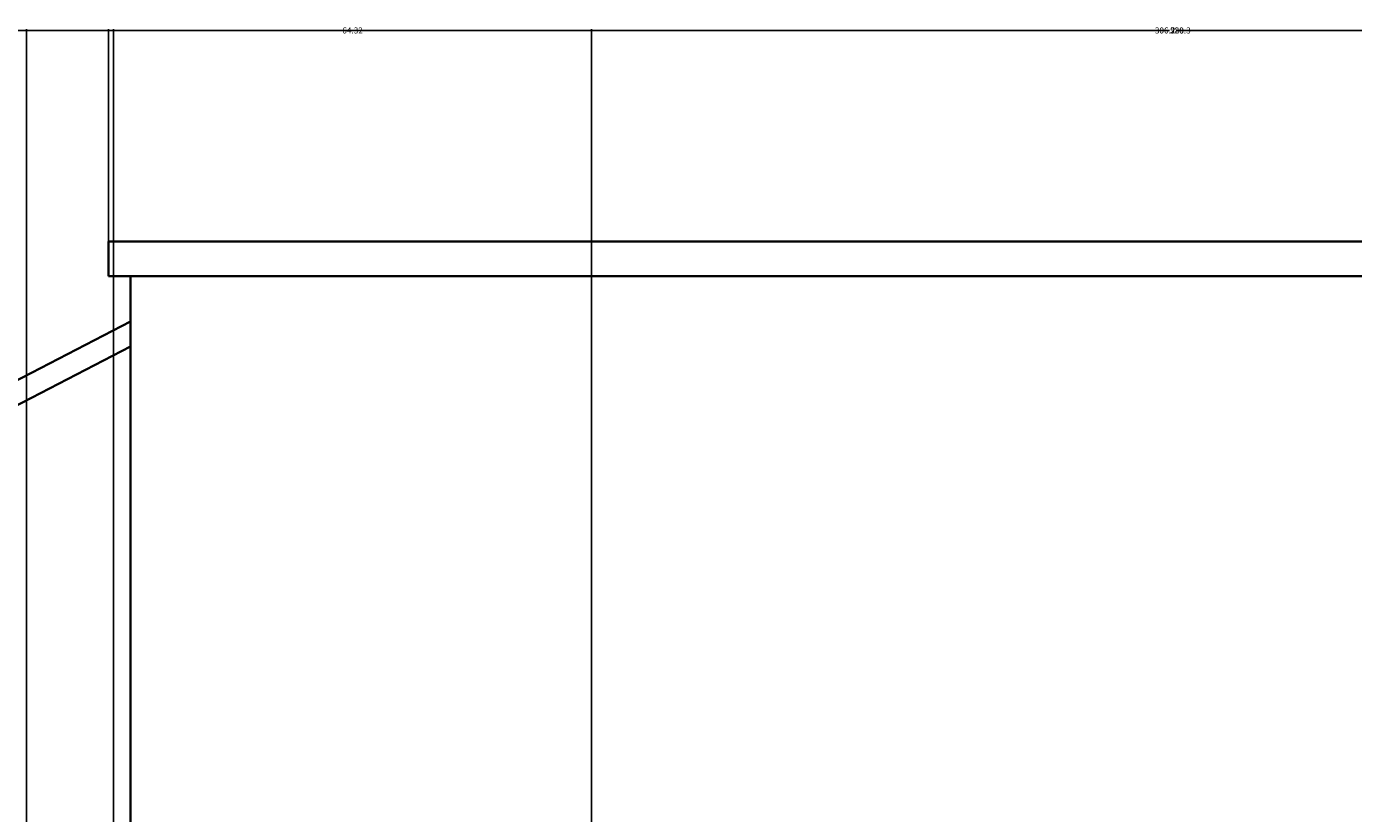
# Model space of a CAD drawing. Units: inches. Extents: x 69 to 650, y -16 to 573.
# Tile 18 of 26: x 205 to 383, y 467 to 573. Entities that reach past the tile are written whole.
import ezdxf

# ---------------------------------------------------------------- set-up
doc = ezdxf.new("R2010")
doc.units = ezdxf.units.IN
doc.header["$MEASUREMENT"] = 0
for name, color, linetype, lineweight in [('A-ANNO-DIMS', 2, 'Continuous', 18), ('A-ROOF', 7, 'Continuous', 35), ('A-WALL', 7, 'Continuous', 35)]:
    doc.layers.add(name, color=color, linetype=linetype, lineweight=lineweight)
doc.styles.get("Standard").update_dxf_attribs({"font": 'arial.ttf'})
doc.dimstyles.get("Standard").update_dxf_attribs({"dimtxt": 0.8125, "dimasz": 0.18, "dimexe": 0.18, "dimexo": 0.0625, "dimgap": 0.09, "dimtad": 0, "dimtih": 1, "dimtoh": 1, "dimdec": 4, "dimzin": 0, "dimdsep": 46, "dimlunit": 4, "dimtxsty": 'Standard', "dimcen": 0.09, "dimadec": 0, "dimazin": 0, "dimtfac": 1, "dimtdec": 4, "dimtofl": 0, "dimtmove": 0, "dimatfit": 3, "dimfxl": 1, "dimtolj": 1, "dimtzin": 0, "dimarcsym": 0})

# ---------------------------------------------------------------- blocks, each defined once
blk = doc.blocks.new('*D19')
at = {"layer": 'A-ANNO-DIMS', "color": 0, "lineweight": -2, "transparency": 16777216}
for p, q in [((99.56, 471.72), (99.56, 572.74)), ((99.74, 572.56), (358.57, 572.56)), ((619.38, 572.56), (360.54, 572.56)), ((619.56, 87.99), (619.56, 572.74))]:
    blk.add_line(p, q, dxfattribs=at)
at = {"layer": 'A-ANNO-DIMS', "color": 0, "transparency": 16777216}
for points in [[(99.74, 572.59), (99.74, 572.53), (99.56, 572.56)], [(619.38, 572.59), (619.38, 572.53), (619.56, 572.56)]]:
    blk.add_solid(points, dxfattribs=at)
at = {"layer": 'Defpoints', "color": 0, "transparency": 16777216}
for p in [(619.56, 572.56), (99.56, 471.66), (619.56, 87.93)]:
    blk.add_point(p, dxfattribs=at)
at = {"layer": 'A-ANNO-DIMS', "color": 0, "transparency": 16777216, "insert": (359.56, 572.56), "char_height": 0.812, "attachment_point": 5}
blk.add_mtext('\\A1;520', dxfattribs=at)
blk = doc.blocks.new('*D45')
at = {"layer": 'A-ANNO-DIMS', "color": 0, "lineweight": -2, "transparency": 16777216}
for p, q in [((216.55, 353.2), (216.55, 572.74)), ((216.73, 572.56), (247.25, 572.56)), ((280.68, 572.56), (250.16, 572.56)), ((280.86, 353.2), (280.86, 572.74))]:
    blk.add_line(p, q, dxfattribs=at)
at = {"layer": 'A-ANNO-DIMS', "color": 0, "transparency": 16777216}
for points in [[(216.73, 572.59), (216.73, 572.53), (216.55, 572.56)], [(280.68, 572.59), (280.68, 572.53), (280.86, 572.56)]]:
    blk.add_solid(points, dxfattribs=at)
at = {"layer": 'Defpoints', "color": 0, "transparency": 16777216}
for p in [(280.86, 572.56), (216.55, 353.14), (280.86, 353.14)]:
    blk.add_point(p, dxfattribs=at)
at = {"layer": 'A-ANNO-DIMS', "color": 0, "transparency": 16777216, "insert": (248.71, 572.56), "char_height": 0.812, "attachment_point": 5}
blk.add_mtext('\\A1;64.32', dxfattribs=at)
blk = doc.blocks.new('*D49')
at = {"layer": 'A-ANNO-DIMS', "color": 0, "lineweight": -2, "transparency": 16777216}
for p, q in [((99.56, 471.72), (99.56, 572.74)), ((99.74, 572.56), (155.98, 572.56)), ((215.7, 572.56), (159.45, 572.56)), ((215.88, 544.22), (215.88, 572.74))]:
    blk.add_line(p, q, dxfattribs=at)
at = {"layer": 'A-ANNO-DIMS', "color": 0, "transparency": 16777216}
for points in [[(99.74, 572.59), (99.74, 572.53), (99.56, 572.56)], [(215.7, 572.59), (215.7, 572.53), (215.88, 572.56)]]:
    blk.add_solid(points, dxfattribs=at)
at = {"layer": 'Defpoints', "color": 0, "transparency": 16777216}
for p in [(215.88, 572.56), (215.88, 544.16), (99.56, 471.66)]:
    blk.add_point(p, dxfattribs=at)
at = {"layer": 'A-ANNO-DIMS', "color": 0, "transparency": 16777216, "insert": (157.72, 572.56), "char_height": 0.812, "attachment_point": 5}
blk.add_mtext('\\A1;116.32', dxfattribs=at)
blk = doc.blocks.new('*D50')
at = {"layer": 'A-ANNO-DIMS', "color": 0, "lineweight": -2, "transparency": 16777216}
for p, q in [((215.88, 544.22), (215.88, 572.74)), ((216.06, 572.56), (358.56, 572.56)), ((504, 572.56), (361.49, 572.56)), ((504.18, 544.22), (504.18, 572.74))]:
    blk.add_line(p, q, dxfattribs=at)
at = {"layer": 'A-ANNO-DIMS', "color": 0, "transparency": 16777216}
for points in [[(216.06, 572.59), (216.06, 572.53), (215.88, 572.56)], [(504, 572.59), (504, 572.53), (504.18, 572.56)]]:
    blk.add_solid(points, dxfattribs=at)
at = {"layer": 'Defpoints', "color": 0, "transparency": 16777216}
for p in [(504.18, 572.56), (215.88, 544.16), (504.18, 544.16)]:
    blk.add_point(p, dxfattribs=at)
at = {"layer": 'A-ANNO-DIMS', "color": 0, "transparency": 16777216, "insert": (360.03, 572.56), "char_height": 0.812, "attachment_point": 5}
blk.add_mtext('\\A1;288.3', dxfattribs=at)
blk = doc.blocks.new('*D62')
at = {"layer": 'A-ANNO-DIMS', "color": 0, "lineweight": -2, "transparency": 16777216}
for p, q in [((204.87, 452.8), (204.87, 572.74)), ((205.05, 572.56), (356.52, 572.56)), ((510.91, 572.56), (359.44, 572.56)), ((511.09, 451.98), (511.09, 572.74))]:
    blk.add_line(p, q, dxfattribs=at)
at = {"layer": 'A-ANNO-DIMS', "color": 0, "transparency": 16777216}
for points in [[(205.05, 572.59), (205.05, 572.53), (204.87, 572.56)], [(510.91, 572.59), (510.91, 572.53), (511.09, 572.56)]]:
    blk.add_solid(points, dxfattribs=at)
at = {"layer": 'Defpoints', "color": 0, "transparency": 16777216}
for p in [(511.09, 572.56), (204.87, 452.74), (511.09, 451.92)]:
    blk.add_point(p, dxfattribs=at)
at = {"layer": 'A-ANNO-DIMS', "color": 0, "transparency": 16777216, "insert": (357.98, 572.56), "char_height": 0.812, "attachment_point": 5}
blk.add_mtext('\\A1;306.2', dxfattribs=at)

msp = doc.modelspace()

# ---------------------------------------------------------------- linework, layer by layer
at = {"layer": 'A-ROOF'}
for p, q in [((215.8767, 539.5075), (215.8767, 544.1573)), ((215.8767, 544.1573), (504.1763, 544.1573)), ((218.848, 539.5075), (215.8767, 539.5075)), ((218.848, 539.5075), (500.263, 539.5075)), ((99.556, 471.6595), (218.848, 533.4142)), ((100.9352, 468.9953), (218.848, 530.036))]:
    msp.add_line(p, q, dxfattribs=at)
at = {"layer": 'A-WALL'}
for p, q in [((218.848, 533.4142), (218.848, 539.5075)), ((218.848, 411.93), (218.848, 533.4142))]:
    msp.add_line(p, q, dxfattribs=at)

# ---------------------------------------------------------------- dimensions: what is measured, and where the dimension line sits
at = {"layer": 'A-ANNO-DIMS'}
for base, p1, p2, override, picture, middle in [((619.555, 572.5573), (99.556, 471.6595), (619.555, 87.93), {"dimdec": 0, "dimlfac": 1, "dimrnd": 0, "dimzin": 0, "dimdsep": 46, "dimlunit": 2}, '*D19', (359.5555, 572.5573)), ((215.8767, 572.5573), (99.556, 471.6595), (215.8767, 544.1573), {"dimdec": 2, "dimlfac": 1, "dimrnd": 0, "dimzin": 0, "dimdsep": 46, "dimlunit": 2}, '*D49', (157.7164, 572.5573)), ((511.0913, 572.5573), (204.8658, 452.7384), (511.0913, 451.9213), {"dimdec": 1, "dimlfac": 1, "dimrnd": 0, "dimzin": 0, "dimdsep": 46, "dimlunit": 2}, '*D62', (357.9786, 572.5573)), ((504.1763, 572.5573), (215.8767, 544.1573), (504.1763, 544.1573), {"dimdec": 1, "dimlfac": 1, "dimrnd": 0, "dimzin": 0, "dimdsep": 46, "dimlunit": 2}, '*D50', (360.0265, 572.5573)), ((280.864, 572.5573), (216.5473, 353.1381), (280.864, 353.1381), {"dimdec": 2, "dimlfac": 1, "dimrnd": 0, "dimzin": 0, "dimdsep": 46, "dimlunit": 2}, '*D45', (248.7057, 572.5573))]:
    dim = msp.add_linear_dim(base=base, p1=p1, p2=p2, dimstyle='Standard', override=override, dxfattribs=at)
    dim.commit()
    dim.dimension.update_dxf_attribs({"geometry": picture, "text_midpoint": middle})

doc.saveas('drawing.dxf')
